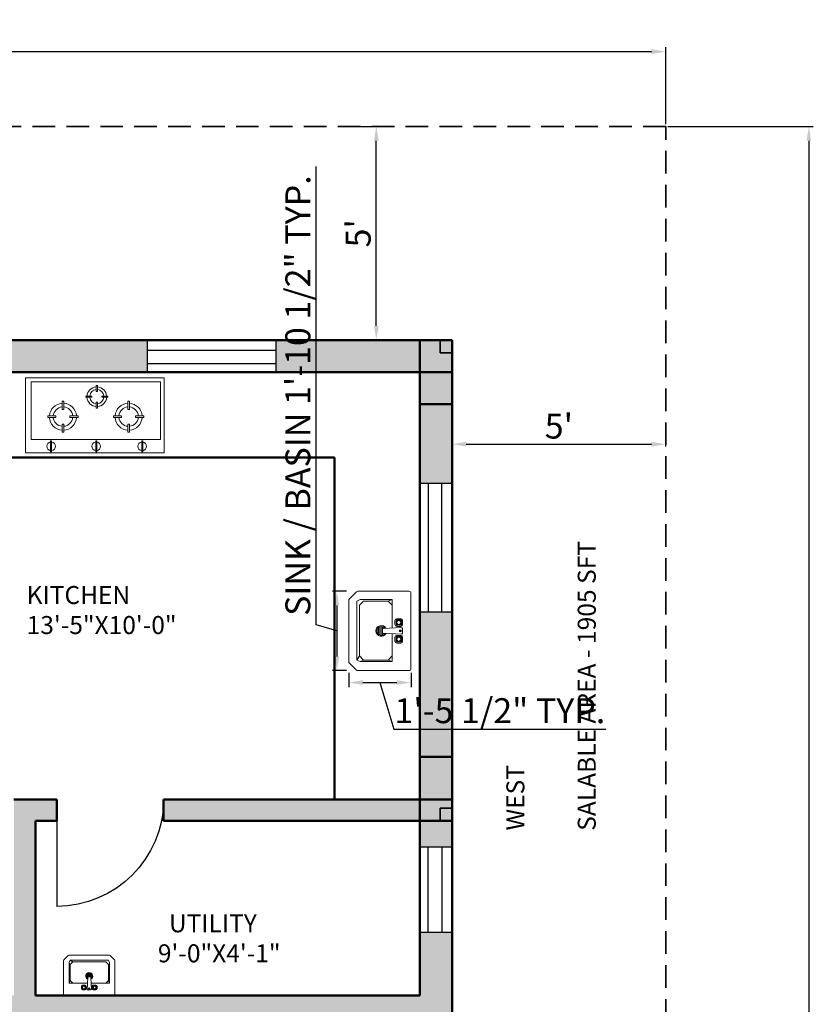
# Model space of a CAD drawing. Units: inches. Extents: x -7 to 1228, y -146 to 1091.
# Tile 88 of 88: x 1006 to 1228, y 814 to 1091. Entities that reach past the tile are written whole.
import ezdxf

# ---------------------------------------------------------------- set-up
doc = ezdxf.new("R2010")
doc.units = ezdxf.units.IN
doc.linetypes.add('DASHED2', pattern=[9.525, 6.35, -3.175])
for name, color, linetype, lineweight in [('A-ANNO-DIMS', 2, 'Continuous', 18), ('A-ANNO-TEXT', 7, 'Continuous', 18), ('A-AREA-IDEN', 7, 'Continuous', 18), ('A-COLS', 6, 'Continuous', 35), ('A-DOOR', 4, 'Continuous', 25), ('A-FURN', 8, 'Continuous', 18), ('A-GLAZ', 175, 'Continuous', 25), ('A-WALL', 7, 'Continuous', 50), ('A-WALL-PATT', 251, 'Continuous', 13), ('C-PROP', 1, 'DASHED2', 35)]:
    doc.layers.add(name, color=color, linetype=linetype, lineweight=lineweight)
doc.styles.get("Standard").update_dxf_attribs({"font": 'arial.ttf'})
doc.dimstyles.new('ISO-25', dxfattribs={"dimtxt": 7, "dimasz": 4, "dimexe": 1.25, "dimexo": 0.625, "dimtad": 1, "dimdec": 1, "dimlunit": 3, "dimtxsty": 'Standard', "dimcen": 2.5, "dimadec": 0, "dimazin": 0, "dimtfac": 1, "dimtdec": 1, "dimtmove": 1, "dimatfit": 3, "dimfxl": 1, "dimarcsym": 0})

# ---------------------------------------------------------------- blocks, each defined once
blk = doc.blocks.new('A$C72243D80')
at = {"ltscale": 1000}
for p, q in [((0, 0), (0, 384.2)), ((0, 384.2), (712, 384.2)), ((29.5, 68.9), (29.5, 363.2)), ((29.5, 363.2), (692.7, 363.2)), ((692.7, 363.2), (692.7, 68.9)), ((712, 384.2), (712, 0)), ((363.5, 314.5), (363.5, 345.1)), ((363.5, 345.1), (369.5, 345.1)), ((369.5, 314.5), (363.5, 314.5)), ((369.5, 345.1), (369.5, 314.5)), ((188.1, 264.2), (188.1, 222.1)), ((196.4, 264.2), (188.1, 264.2)), ((196.4, 222.1), (196.4, 264.2)), ((309.4, 291), (340, 291)), ((309.4, 285), (309.4, 291)), ((340, 285), (309.4, 285)), ((340, 291), (340, 285)), ((363.5, 260), (363.5, 229.4)), ((369.5, 260), (363.5, 260)), ((369.5, 229.4), (369.5, 260)), ((392.3, 291), (392.3, 285)), ((422.9, 291), (392.3, 291)), ((392.3, 285), (422.9, 285)), ((422.9, 285), (422.9, 291)), ((525.9, 222.1), (525.9, 264.2)), ((525.9, 264.2), (534.1, 264.2)), ((534.1, 264.2), (534.1, 222.1)), ((188.1, 222.1), (196.4, 222.1)), ((363.5, 229.4), (369.5, 229.4)), ((534.1, 222.1), (525.9, 222.1)), ((114.7, 189.8), (156.8, 189.8)), ((114.7, 181.6), (114.7, 189.8)), ((156.8, 181.6), (114.7, 181.6)), ((156.8, 189.8), (156.8, 181.6)), ((228.6, 189.8), (228.6, 181.6)), ((270.7, 189.8), (228.6, 189.8)), ((228.6, 181.6), (270.7, 181.6)), ((270.7, 181.6), (270.7, 189.8)), ((451.5, 189.8), (493.6, 189.8)), ((451.5, 181.6), (451.5, 189.8)), ((493.6, 181.6), (451.5, 181.6)), ((493.6, 189.8), (493.6, 181.6)), ((565.5, 189.8), (565.5, 181.6)), ((607.6, 189.8), (565.5, 189.8)), ((565.5, 181.6), (607.6, 181.6)), ((607.6, 181.6), (607.6, 189.8)), ((188.1, 147.2), (196.4, 147.2)), ((188.1, 105.1), (188.1, 147.2)), ((196.4, 105.1), (188.1, 105.1)), ((196.4, 147.2), (196.4, 105.1)), ((525.9, 147.2), (525.9, 105.1)), ((534.1, 147.2), (525.9, 147.2)), ((525.9, 105.1), (534.1, 105.1)), ((534.1, 105.1), (534.1, 147.2)), ((692.7, 68.9), (29.5, 68.9)), ((129.6, 61.1), (129.6, 5)), ((134.4, 61.1), (129.6, 61.1)), ((134.4, 5), (134.4, 61.1)), ((360.9, 5), (360.9, 61.1)), ((360.9, 61.1), (365.7, 61.1)), ((365.7, 61.1), (365.7, 5)), ((597, 5), (597, 61.1)), ((597, 61.1), (601.8, 61.1)), ((601.8, 61.1), (601.8, 5)), ((712, 0), (0, 0)), ((129.6, 5), (134.4, 5)), ((365.7, 5), (360.9, 5)), ((601.8, 5), (597, 5))]:
    blk.add_line(p, q, dxfattribs=at)
for centre, radius, start, end in [((366.2, 287.2), 50.3, 93.0344, 175.7271), ((366.1, 287.8), 36.3, 94.0374, 175.0142), ((366.2, 287.2), 50.3, 4.2729, 86.1838), ((366.1, 287.8), 36.3, 4.9858, 84.5356), ((192.7, 184.7), 69.2, 93.8162, 175.7271), ((192.7, 184.7), 69.2, 4.2729, 86.9656), ((366.2, 287.2), 50.3, 182.5783, 266.9656), ((366.1, 287.8), 36.3, 184.5153, 265.9626), ((366.1, 287.8), 36.3, 275.4644, 355.4847), ((366.2, 287.2), 50.3, 273.8162, 357.4217), ((529.5, 184.7), 69.2, 93.0344, 175.7271), ((529.5, 184.7), 69.2, 4.2729, 86.1838), ((192.9, 185.5), 49.9, 95.4644, 175.0142), ((192.9, 185.5), 49.9, 4.9858, 85.9626), ((529.4, 185.5), 49.9, 94.0374, 175.0142), ((529.4, 185.5), 49.9, 4.9858, 84.5356), ((192.7, 184.7), 69.2, 182.5783, 266.1838), ((192.9, 185.5), 49.9, 184.5153, 264.5356), ((192.9, 185.5), 49.9, 274.0374, 355.4847), ((192.7, 184.7), 69.2, 273.0344, 357.4217), ((529.5, 184.7), 69.2, 182.5783, 266.9656), ((529.4, 185.5), 49.9, 184.5153, 265.9626), ((529.5, 184.7), 69.2, 273.8162, 357.4217), ((529.4, 185.5), 49.9, 275.4644, 355.4847), ((132.3, 33.2), 22.5, 96.7453, 263.2547), ((132.3, 33.2), 22.5, 275.4789, 84.5211), ((363.1, 33.2), 22.5, 95.4789, 264.5211), ((363.1, 33.2), 22.5, 276.7453, 83.2547), ((599.2, 33.2), 22.5, 95.4789, 264.5211), ((599.2, 33.2), 22.5, 276.7453, 83.2547)]:
    blk.add_arc(centre, radius, start, end, dxfattribs=at)
blk = doc.blocks.new('A$C4CB854FF')
for p, q in [((0, 0.3675), (0, 0.0552)), ((0.4725, 0.38), (0.0125, 0.38)), ((0.485, 0.0552), (0.485, 0.3675)), ((0.1677, 0.2932), (0.1677, 0.318)), ((0.1745, 0.2919), (0.1745, 0.3194)), ((0.1773, 0.3221), (0.2048, 0.3221)), ((0.1787, 0.329), (0.2034, 0.329)), ((0.2075, 0.3194), (0.2075, 0.2919)), ((0.2144, 0.318), (0.2144, 0.2932)), ((0.2279, 0.2104), (0.2213, 0.3235)), ((0.2337, 0.329), (0.2502, 0.329)), ((0.2625, 0.3235), (0.256, 0.2104)), ((0.2694, 0.318), (0.2694, 0.2932)), ((0.2763, 0.3194), (0.2763, 0.2919)), ((0.3065, 0.3221), (0.279, 0.3221)), ((0.3052, 0.329), (0.2804, 0.329)), ((0.3093, 0.2919), (0.3093, 0.3194)), ((0.3162, 0.2932), (0.3162, 0.318)), ((0.05, 0.265), (0.2247, 0.265)), ((0.06, 0.24), (0.05, 0.265)), ((0.05, 0.07), (0.05, 0.265)), ((0.085, 0.265), (0.06, 0.24)), ((0.2048, 0.2891), (0.1773, 0.2891)), ((0.2034, 0.2822), (0.1787, 0.2822)), ((0.2591, 0.265), (0.43, 0.265)), ((0.279, 0.2891), (0.3065, 0.2891)), ((0.2804, 0.2822), (0.3052, 0.2822)), ((0.395, 0.265), (0.42, 0.24)), ((0.42, 0.24), (0.43, 0.265)), ((0.43, 0.07), (0.43, 0.265)), ((0.06, 0.24), (0.06, 0.09)), ((0.2152, 0.1984), (0.2694, 0.1984)), ((0.2297, 0.2066), (0.2165, 0.2066)), ((0.2681, 0.1901), (0.2165, 0.1901)), ((0.2272, 0.2149), (0.2208, 0.2149)), ((0.2638, 0.1819), (0.2208, 0.1819)), ((0.2505, 0.2052), (0.2334, 0.2052)), ((0.2681, 0.2066), (0.2541, 0.2066)), ((0.2638, 0.2149), (0.2566, 0.2149)), ((0.42, 0.24), (0.42, 0.09)), ((0.2533, 0.1736), (0.2313, 0.1736)), ((0.05, 0.07), (0.06, 0.05)), ((0.06, 0.09), (0.085, 0.065)), ((0.085, 0.065), (0.395, 0.065)), ((0.42, 0.09), (0.395, 0.065)), ((0.395, 0.065), (0.42, 0.05)), ((0.42, 0.09), (0.43, 0.07)), ((0.43, 0.07), (0.42, 0.05)), ((0.0037, 0.0463), (0.0463, 0.0037)), ((0.42, 0.05), (0.06, 0.05)), ((0.4387, 0.0037), (0.4813, 0.0463)), ((0.0552, 0), (0.4298, 0))]:
    blk.add_line(p, q)
for centre, radius in [((0.191, 0.3056), 0.0165), ((0.191, 0.3056), 0.0127), ((0.2419, 0.3152), 0.00688), ((0.2419, 0.3152), 0.00344), ((0.2928, 0.3056), 0.0165), ((0.2928, 0.3056), 0.0127)]:
    blk.add_circle(centre, radius)
for centre, radius, start, end in [((0.0125, 0.3675), 0.0125, 90, 180), ((0.4725, 0.3675), 0.0125, 0, 90), ((0.1787, 0.318), 0.011, 90, 180), ((0.1773, 0.3194), 0.00275, 90, 180), ((0.2034, 0.318), 0.011, 0, 90), ((0.2048, 0.3194), 0.00275, 360, 90), ((0.2329, 0.314), 0.015, 87.19754, 140.72744), ((0.2509, 0.314), 0.015, 39.27256, 92.80246), ((0.2804, 0.318), 0.011, 90, 180), ((0.279, 0.3194), 0.00275, 90, 180), ((0.3052, 0.318), 0.011, 0, 90), ((0.3065, 0.3194), 0.00275, 360, 90), ((0.1787, 0.2932), 0.011, 180, 270), ((0.1773, 0.2919), 0.00275, 180, 270), ((0.2034, 0.2932), 0.011, 270, 0), ((0.2048, 0.2919), 0.00275, 270, 0), ((0.2804, 0.2932), 0.011, 180, 270), ((0.279, 0.2919), 0.00275, 180, 270), ((0.3052, 0.2932), 0.011, 270, 360), ((0.3065, 0.2919), 0.00275, 270, 0), ((0.2423, 0.1984), 0.033, 118.68833, 62.86857), ((0.2423, 0.1984), 0.0271, 124.77581, 57.22467), ((0.2334, 0.2107), 0.0055, 183.3274, 270), ((0.2505, 0.2107), 0.0055, 270, 356.6726), ((0.0125, 0.0552), 0.0125, 180, 225), ((0.0552, 0.0125), 0.0125, 225, 270), ((0.4298, 0.0125), 0.0125, 270, 315), ((0.4725, 0.0552), 0.0125, 315, 0)]:
    blk.add_arc(centre, radius, start, end)
blk = doc.blocks.new('*D7')
at = {"layer": 'A-ANNO-DIMS', "color": 0, "lineweight": -2, "transparency": 16777216}
for p, q in [((1099.01, 1061), (1106.99, 1061)), ((1105.74, 1005), (1105.74, 1057)), ((1099.01, 1001), (1106.99, 1001))]:
    blk.add_line(p, q, dxfattribs=at)
at = {"layer": 'A-ANNO-DIMS', "color": 0, "transparency": 16777216}
for points in [[(1105.08, 1057), (1106.41, 1057), (1105.74, 1061)], [(1105.08, 1005), (1106.41, 1005), (1105.74, 1001)]]:
    blk.add_solid(points, dxfattribs=at)
at = {"layer": 'Defpoints', "color": 0, "transparency": 16777216}
for p in [(1098.39, 1061), (1105.74, 1061), (1098.39, 1001)]:
    blk.add_point(p, dxfattribs=at)
at = {"layer": 'A-ANNO-DIMS', "color": 0, "transparency": 16777216, "insert": (1101.56, 1031), "char_height": 7, "attachment_point": 5, "rotation": 90}
blk.add_mtext("5'", dxfattribs=at)
blk = doc.blocks.new('*D8')
at = {"layer": 'A-ANNO-DIMS', "color": 0, "lineweight": -2, "transparency": 16777216}
for p, q in [((1127, 971.1), (1127, 973.02)), ((1131, 971.77), (1183, 971.77)), ((1187, 971.1), (1187, 973.02))]:
    blk.add_line(p, q, dxfattribs=at)
at = {"layer": 'A-ANNO-DIMS', "color": 0, "transparency": 16777216}
for points in [[(1131, 972.44), (1131, 971.1), (1127, 971.77)], [(1183, 972.44), (1183, 971.1), (1187, 971.77)]]:
    blk.add_solid(points, dxfattribs=at)
at = {"layer": 'Defpoints', "color": 0, "transparency": 16777216}
for p in [(1127, 970.48), (1187, 971.77), (1187, 970.48)]:
    blk.add_point(p, dxfattribs=at)
at = {"layer": 'A-ANNO-DIMS', "color": 0, "transparency": 16777216, "insert": (1157, 975.95), "char_height": 7, "attachment_point": 5}
blk.add_mtext("5'", dxfattribs=at)
blk = doc.blocks.new('*D11')
at = {"layer": 'A-ANNO-DIMS', "color": 0, "lineweight": -2, "transparency": 16777216}
for p, q in [((0, 1061.62), (0, 1083.25)), ((4, 1082), (1183, 1082)), ((1187, 1061.62), (1187, 1083.25))]:
    blk.add_line(p, q, dxfattribs=at)
at = {"layer": 'A-ANNO-DIMS', "color": 0, "transparency": 16777216}
for points in [[(4, 1082.67), (4, 1081.33), (0, 1082)], [(1183, 1082.67), (1183, 1081.33), (1187, 1082)]]:
    blk.add_solid(points, dxfattribs=at)
at = {"layer": 'Defpoints', "color": 0, "transparency": 16777216}
for p in [(1187, 1082), (0, 1061), (1187, 1061)]:
    blk.add_point(p, dxfattribs=at)
at = {"layer": 'A-ANNO-DIMS', "color": 0, "transparency": 16777216, "insert": (593.5, 1086.2), "char_height": 7, "attachment_point": 5}
blk.add_mtext('98\'-11"', dxfattribs=at)
blk = doc.blocks.new('*D12')
at = {"layer": 'A-ANNO-DIMS', "color": 0, "lineweight": -2, "transparency": 16777216}
for p, q in [((1187.62, 1061), (1228.45, 1061)), ((1227.2, 1057), (1227.2, 4)), ((1187.62, 0), (1228.45, 0))]:
    blk.add_line(p, q, dxfattribs=at)
at = {"layer": 'A-ANNO-DIMS', "color": 0, "transparency": 16777216}
for points in [[(1226.53, 1057), (1227.86, 1057), (1227.2, 1061)], [(1226.53, 4), (1227.86, 4), (1227.2, 0)]]:
    blk.add_solid(points, dxfattribs=at)
at = {"layer": 'Defpoints', "color": 0, "transparency": 16777216}
for p in [(1187, 1061), (1187, 0), (1227.2, 0)]:
    blk.add_point(p, dxfattribs=at)
at = {"layer": 'A-ANNO-DIMS', "color": 0, "transparency": 16777216, "insert": (1223, 530.5), "char_height": 7, "attachment_point": 5, "rotation": 90}
blk.add_mtext('88\'-5"', dxfattribs=at)
blk = doc.blocks.new('WIN-36')
for p, q in [((0, 36), (0, 0)), ((9, 36), (0, 36)), ((2.34, 36), (2.34, 0)), ((6.14, 0), (6.14, 36)), ((9, 0), (9, 36)), ((0, 0), (9, 0)), ((2.34, 0), (6.14, 0))]:
    blk.add_line(p, q)
blk = doc.blocks.new('WIN-24')
for p, q in [((0, 0), (0, 24)), ((0, 24), (9, 24)), ((2.34, 0), (2.34, 24)), ((2.34, 24), (6.14, 24)), ((6.14, 24), (6.14, 0)), ((9, 24), (9, 0)), ((9, 0), (0, 0))]:
    blk.add_line(p, q)
blk = doc.blocks.new('DOOR-750')
blk.add_line((30, 30), (30, 0))
blk.add_arc((30, 30), 30, 180, 270)
blk = doc.blocks.new('*D30')
at = {"layer": 'A-ANNO-DIMS', "color": 0, "lineweight": -2, "transparency": 16777216}
for p, q in [((1088.85, 921.08), (1088.85, 1049.76)), ((1097.38, 930.49), (1093.41, 930.49)), ((1094.66, 926.49), (1094.66, 912.19)), ((1094.66, 919.34), (1088.85, 921.08)), ((1097.38, 908.19), (1093.41, 908.19))]:
    blk.add_line(p, q, dxfattribs=at)
at = {"layer": 'A-ANNO-DIMS', "color": 0, "transparency": 16777216}
for points in [[(1093.99, 926.49), (1095.32, 926.49), (1094.66, 930.49)], [(1093.99, 912.19), (1095.32, 912.19), (1094.66, 908.19)]]:
    blk.add_solid(points, dxfattribs=at)
at = {"layer": 'Defpoints', "color": 0, "transparency": 16777216}
for p in [(1098, 930.49), (1094.66, 908.19), (1098, 908.19)]:
    blk.add_point(p, dxfattribs=at)
at = {"layer": 'A-ANNO-DIMS', "color": 0, "transparency": 16777216, "insert": (1084.61, 985.42), "char_height": 7, "attachment_point": 5, "rotation": 90}
blk.add_mtext('SINK / BASIN 1\'-10 1/2" TYP.', dxfattribs=at)
blk = doc.blocks.new('*D31')
at = {"layer": 'A-ANNO-DIMS', "color": 0, "lineweight": -2, "transparency": 16777216}
for p, q in [((1098, 907.56), (1098, 903.59)), ((1115.48, 907.56), (1115.48, 903.59)), ((1102, 904.84), (1111.48, 904.84)), ((1106.74, 904.84), (1110.66, 891.8)), ((1110.66, 891.8), (1170.23, 891.8))]:
    blk.add_line(p, q, dxfattribs=at)
at = {"layer": 'A-ANNO-DIMS', "color": 0, "transparency": 16777216}
for points in [[(1102, 905.51), (1102, 904.18), (1098, 904.84)], [(1111.48, 905.51), (1111.48, 904.18), (1115.48, 904.84)]]:
    blk.add_solid(points, dxfattribs=at)
at = {"layer": 'Defpoints', "color": 0, "transparency": 16777216}
for p in [(1098, 908.19), (1115.48, 908.19), (1115.48, 904.84)]:
    blk.add_point(p, dxfattribs=at)
at = {"layer": 'A-ANNO-DIMS', "color": 0, "transparency": 16777216, "insert": (1140.44, 896.04), "char_height": 7, "attachment_point": 5}
blk.add_mtext('1\'-5 1/2" TYP.', dxfattribs=at)

msp = doc.modelspace()

# ---------------------------------------------------------------- hatches: boundary and pattern name
at = {"layer": 'A-COLS'}
h = msp.add_hatch(color=256, dxfattribs=at)
h.dxf.hatch_style = 1
h.paths.add_polyline_path([(1127, 997.45), (1123.71, 997.45), (1123.71, 1001), (1118, 1001), (1118, 983), (1127, 983)])
h = msp.add_hatch(color=256, dxfattribs=at)
h.dxf.hatch_style = 1
h.paths.add_polyline_path([(1127, 997.45), (1127, 1001), (1123.71, 1001), (1123.71, 997.45)])
h = msp.add_hatch(color=256, dxfattribs=at)
h.dxf.hatch_style = 1
h.paths.add_polyline_path([(1127, 884), (1118, 884), (1118, 866), (1123.71, 866), (1123.71, 869.55), (1127, 869.55)])
h = msp.add_hatch(color=256, dxfattribs=at)
h.dxf.hatch_style = 1
h.paths.add_polyline_path([(1123.71, 869.55), (1123.71, 866), (1127, 866), (1127, 869.55)])
at = {"layer": 'A-WALL-PATT'}
h = msp.add_hatch(color=256, dxfattribs=at)
h.dxf.hatch_style = 1
h.paths.add_polyline_path([(69, 568), (60, 568), (60, 493), (63.29, 493), (69, 493)])
h.paths.add_polyline_path([(69, 662.41), (60, 662.41), (60, 586), (69, 586)], flags=17)
h.paths.add_polyline_path([(69, 723), (184, 723), (184, 734), (179, 734), (179, 728), (69, 728), (69, 741.62), (60, 741.62), (60, 698.41), (69, 698.41)], flags=17)
h.paths.add_polyline_path([(69, 782), (231, 782), (231, 728), (231, 723), (231, 586), (236, 586), (236, 787), (69, 787), (69, 800.13), (60, 800.13), (60, 765.62), (69, 765.62)])
h.paths.add_polyline_path([(184, 842), (189, 842), (189, 848), (173, 848), (173, 842), (179, 842), (179, 787), (184, 787)])
h.paths.add_polyline_path([(118.22, 69), (69, 69), (69, 60), (118.22, 60)])
h.paths.add_polyline_path([(227, 69), (154.22, 69), (154.22, 60), (227, 60)])
h.paths.add_polyline_path([(236, 60), (232.71, 60), (227, 60), (227, 36), (236, 36)])
h.paths.add_polyline_path([(389, 60), (380, 60), (380, 36), (389, 36)])
h.paths.add_polyline_path([(384, 181), (380, 181), (380, 115), (380, 78), (384, 78)])
h.paths.add_polyline_path([(380, 115), (334.55, 115), (334.55, 109), (380, 109)])
h.paths.add_polyline_path([(274.55, 115), (236, 115), (236, 201), (232.71, 201), (231, 201), (231, 78), (236, 78), (236, 109), (274.55, 109)])
h.paths.add_polyline_path([(69, 123), (60, 123), (60, 78), (69, 78)])
h.paths.add_polyline_path([(69, 201), (60, 201), (60, 159), (69, 159)])
h.paths.add_polyline_path([(143, 219), (69, 219), (69, 213), (143, 213)], flags=17)
h.paths.add_polyline_path([(189, 219), (184, 219), (184, 274), (231, 274), (231, 219), (236, 219), (236, 279), (184, 279), (184, 297), (179, 297), (179, 279), (69, 279), (69, 290.91), (60, 290.91), (60, 262.18), (69, 262.18), (69, 274), (179, 274), (179, 219), (173, 219), (173, 213), (189, 213)])
h.paths.add_polyline_path([(69, 238.18), (60, 238.18), (60, 219), (69, 219)], flags=17)
h.paths.add_polyline_path([(69, 333), (60, 333), (60, 314.91), (69, 314.91), (69, 316.96)])
h.paths.add_polyline_path([(190, 338), (184, 338), (69, 338), (69, 333), (179, 333), (179, 327), (184, 327), (184, 333.02), (190, 333.05)])
h.paths.add_polyline_path([(69, 386.81), (60, 386.81), (60, 351), (69, 351)])
h.paths.add_polyline_path([(69, 475), (60, 475), (60, 422.81), (69, 422.81)])
h.paths.add_polyline_path([(236, 475), (231, 475), (231, 351.24), (236, 351.24)])
h.paths.add_polyline_path([(384, 475), (380, 475), (380, 362), (384, 362)])
h.paths.add_polyline_path([(547, 307), (439, 307), (439, 356), (445, 356), (445, 362), (433, 362), (433, 307), (380, 307), (380, 244), (380, 241), (384, 241), (384, 301), (433, 301), (433, 277), (439, 277), (439, 301), (547, 301)])
h.paths.add_polyline_path([(547, 241), (439, 241), (439, 247), (433, 247), (433, 235), (547, 235)])
h.paths.add_polyline_path([(450, 69), (440.29, 69), (424.89, 69), (389, 69), (389, 60), (450, 60)])
h.paths.add_polyline_path([(547, 69), (486, 69), (486, 60), (547, 60)])
h.paths.add_polyline_path([(556, 148.27), (547, 148.27), (547, 78), (556, 78)])
h.paths.add_polyline_path([(556, 223), (547, 223), (547, 195), (547, 184.27), (556, 184.27)])
h.paths.add_polyline_path([(556, 311.19), (547, 311.19), (547, 273.08), (556, 273.08)])
h.paths.add_polyline_path([(556, 344), (552.71, 344), (547, 344), (547, 335.19), (556, 335.19)])
h.paths.add_polyline_path([(556, 249.08), (547, 249.08), (547, 241), (556, 241)])
h.paths.add_polyline_path([(547, 362), (475, 362), (475, 356), (547, 356)], flags=0)
h.paths.add_polyline_path([(556, 399.62), (547, 399.62), (547, 362), (556, 362)])
h.paths.add_polyline_path([(556, 475), (547, 475), (547, 435.62), (556, 435.62)])
h.paths.add_polyline_path([(547, 493), (389, 493), (389, 487), (547, 487)])
h.paths.add_polyline_path([(380, 493), (278, 493), (278, 487), (380, 487)])
h.paths.add_polyline_path([(227, 493), (69, 493), (69, 487), (227, 487)])
h.paths.add_polyline_path([(643, 122.44), (634, 122.44), (634, 78), (643, 78)])
h.paths.add_polyline_path([(702.5, 69), (692.79, 69), (677.39, 69), (643, 69), (643, 60), (702.5, 60)])
h.paths.add_polyline_path([(798, 69), (738.5, 69), (738.5, 60), (798, 60)])
h.paths.add_polyline_path([(807, 60), (803.71, 60), (798, 60), (798, 36), (807, 36)])
h.paths.add_polyline_path([(807, 109), (846.75, 109), (846.75, 115), (807, 115), (807, 159), (802, 159), (802, 78), (807, 78)])
h.paths.add_polyline_path([(807, 201), (802, 201), (802, 195), (807, 195)])
h.paths.add_polyline_path([(643, 201), (634, 201), (634, 158.44), (643, 158.44)])
h.paths.add_polyline_path([(756, 225), (751, 225), (751, 219), (643, 219), (643, 213), (756, 213)])
h.paths.add_polyline_path([(643, 240.85), (634, 240.85), (634, 219), (643, 219)])
h.paths.add_polyline_path([(643, 274), (643, 288.63), (634, 288.63), (634, 264.85), (643, 264.85)])
h.paths.add_polyline_path([(802, 279), (756, 279), (756, 297), (751, 297), (751, 279), (643, 279), (643, 274), (751, 274), (751, 255), (756, 255), (756, 274), (802, 274)])
h.paths.add_polyline_path([(807, 333), (803.71, 333), (802, 333), (802, 279), (802, 274), (802, 219), (807, 219)])
h.paths.add_polyline_path([(956, 182), (951, 182), (951, 115), (906.75, 115), (906.75, 109), (951, 109), (951, 78), (956, 78)])
h.paths.add_polyline_path([(960, 60), (951, 60), (951, 36), (960, 36)])
h.paths.add_polyline_path([(1021, 69), (1005.78, 69), (960, 69), (960, 60), (1021, 60)])
h.paths.add_polyline_path([(956, 224), (951, 224), (951, 218), (956, 218)])
h.paths.add_polyline_path([(956, 302), (1004, 302), (1004, 278), (1010, 278), (1010, 302), (1118, 302), (1118, 290.81), (1127, 290.81), (1127, 326.97), (1118, 326.97), (1118, 320.97), (1118, 307), (1010, 307), (1010, 356), (1016, 356), (1016, 362), (1004, 362), (1004, 307), (951, 307), (951, 244), (951, 242), (954.29, 242), (956, 242)])
h.paths.add_polyline_path([(643, 333), (634, 333), (634, 312.63), (643, 312.63), (643, 316.96)])
h.paths.add_polyline_path([(756, 338), (643, 338), (643, 333), (751, 333), (751, 327), (756, 327)])
h.paths.add_polyline_path([(643, 388), (634, 388), (634, 351), (643, 351)])
h.paths.add_polyline_path([(807, 357), (802, 357), (802, 351), (807, 351)])
h.paths.add_polyline_path([(807, 475), (802, 475), (802, 393), (807, 393)])
h.paths.add_polyline_path([(643, 475), (634, 475), (634, 424), (643, 424)])
h.paths.add_polyline_path([(798, 493), (643, 493), (643, 487), (798, 487)])
h.paths.add_polyline_path([(634, 493), (556, 493), (556, 487), (634, 487)])
h.paths.add_polyline_path([(813, 493), (807, 493), (807, 487), (813, 487)])
h.paths.add_polyline_path([(951, 493), (849, 493), (849, 487), (951, 487)])
h.paths.add_polyline_path([(956, 484), (951, 484), (951, 374), (956, 374)])
h.paths.add_polyline_path([(1109, 493), (969, 493), (969, 487), (1109, 487)])
h.paths.add_polyline_path([(1127, 484), (1118, 484), (1118, 450.64), (1127, 450.64)])
h.paths.add_polyline_path([(1127, 414.64), (1118, 414.64), (1118, 365), (1127, 365)])
h.paths.add_polyline_path([(1109, 362), (1046, 362), (1046, 356), (1109, 356)], flags=17)
h.paths.add_polyline_path([(1127, 356), (1123.45, 356), (1118, 356), (1118, 350.97), (1127, 350.97)], flags=0)
h.paths.add_polyline_path([(1127, 266.81), (1118, 266.81), (1118, 262.36), (1118, 242), (1127, 242)], flags=17)
h.paths.add_polyline_path([(1118, 242), (1010, 242), (1010, 248), (1004, 248), (1004, 237), (1118, 237)])
h.paths.add_polyline_path([(1127, 224), (1118, 224), (1118, 170), (1127, 170)])
h.paths.add_polyline_path([(1127, 134), (1118, 134), (1118, 78), (1127, 78)])
h.paths.add_polyline_path([(1118, 69), (1057, 69), (1057, 60), (1118, 60)])
h.paths.add_polyline_path([(227, 571.55), (227, 574), (69, 574), (69, 568), (227, 568)])
h.paths.add_polyline_path([(380, 571.55), (380, 574), (278, 574), (278, 568), (380, 568)])
h.paths.add_polyline_path([(242, 574), (236, 574), (236, 568), (242, 568)])
h.paths.add_polyline_path([(547, 571.55), (547, 574), (389, 574), (389, 568), (547, 568)])
h.paths.add_polyline_path([(384, 733), (380, 733), (380, 586), (384, 586)])
h.paths.add_polyline_path([(556, 646), (634, 646), (634, 655), (547, 655), (547, 586), (556, 586)])
h.paths.add_polyline_path([(634, 574), (556, 574), (556, 568), (634, 568)])
h.paths.add_polyline_path([(643, 655), (634, 655), (634, 586), (643, 586)])
h.paths.add_polyline_path([(798, 574), (643, 574), (643, 568), (798, 568)])
h.paths.add_polyline_path([(643, 663.85), (634, 663.85), (634, 655), (643, 655)])
h.paths.add_polyline_path([(556, 676.97), (547, 676.97), (547, 655), (556, 655)])
h.paths.add_polyline_path([(556, 733), (547, 733), (547, 712.97), (556, 712.97)])
h.paths.add_polyline_path([(643, 710), (634, 710), (634, 699.85), (643, 699.85)])
h.paths.add_polyline_path([(807, 668), (802, 668), (802, 586), (807, 586)])
h.paths.add_polyline_path([(951, 574), (849, 574), (849, 568), (951, 568)])
h.paths.add_polyline_path([(956, 691), (951, 691), (951, 577), (956, 577)])
h.paths.add_polyline_path([(1109, 574), (969, 574), (969, 568), (1109, 568)])
h.paths.add_polyline_path([(1127, 643.4), (1118, 643.4), (1118, 577), (1127, 577)])
h.paths.add_polyline_path([(1127, 568), (1123.45, 568), (1118, 568), (1118, 493), (1127, 493)])
h.paths.add_polyline_path([(1127, 733), (1118, 733), (1118, 679.4), (1127, 679.4)])
h.paths.add_polyline_path([(1127, 777.35), (1118, 777.35), (1118, 770.04), (1118, 751), (1127, 751)], flags=17)
h.paths.add_polyline_path([(1118, 751), (1010, 751), (1010, 757), (1004, 757), (1004, 745), (1118, 745)])
h.paths.add_polyline_path([(956, 811), (1004, 811), (1004, 787), (1010, 787), (1010, 811), (1017.87, 811), (1017.87, 811.63, -0.414214), (1018.25, 812), (1031.98, 812, -0.414214), (1032.35, 811.63), (1032.35, 811), (1118, 811), (1118, 801.35), (1127, 801.35), (1127, 834.69), (1118, 834.69), (1118, 830.24), (1118, 817), (1010, 817), (1010, 866), (1016, 866), (1016, 872), (1004, 872), (1004, 817), (956, 817), (956, 866), (951, 866), (951, 751), (954.29, 751), (956, 751)])
h.paths.add_polyline_path([(1118, 872), (1046, 872), (1046, 866), (1118, 866)], flags=17)
h.paths.add_polyline_path([(1127, 924.71), (1118, 924.71), (1118, 884), (1127, 884)])
h.paths.add_polyline_path([(1127, 866), (1123.71, 866), (1118, 866), (1118, 858.69), (1127, 858.69)], flags=17)
h.paths.add_polyline_path([(956, 983), (951, 983), (951, 952), (807, 952), (807, 983), (802, 983), (802, 902), (807, 902), (807, 946), (951, 946), (951, 884), (956, 884)])
h.paths.add_polyline_path([(807, 842), (802, 842), (802, 787), (756, 787), (756, 806), (751, 806), (751, 787), (643, 787), (643, 782), (751, 782), (751, 764), (756, 764), (756, 782), (802, 782), (802, 728), (807, 728)])
h.paths.add_polyline_path([(756, 848), (643, 848), (643, 842), (751, 842), (751, 836), (756, 836)])
h.paths.add_polyline_path([(756, 734), (751, 734), (751, 728), (643, 728), (643, 723), (756, 723)])
h.paths.add_polyline_path([(643, 749.79), (634, 749.79), (634, 728), (637.29, 728), (643, 728)])
h.paths.add_polyline_path([(643, 805.41), (634, 805.41), (634, 773.79), (643, 773.79)])
h.paths.add_polyline_path([(643, 896.66), (634, 896.66), (634, 860), (637.29, 860), (643, 860)])
h.paths.add_polyline_path([(643, 842), (634, 842), (634, 829.41), (643, 829.41)])
h.paths.add_polyline_path([(643, 983), (634, 983), (634, 932.66), (643, 932.66)])
h.paths.add_polyline_path([(1127, 983), (1118, 983), (1118, 960.71), (1127, 960.71)])
h.paths.add_polyline_path([(1118, 1001), (1077.53, 1001), (1077.53, 992), (1118, 992)])
h.paths.add_polyline_path([(1041.53, 1001), (960, 1001), (960, 992), (1041.53, 992)])
h.paths.add_polyline_path([(960, 1025), (951, 1025), (951, 1001), (954.29, 1001), (960, 1001)])
h.paths.add_polyline_path([(807, 1025), (798, 1025), (798, 1001), (807, 1001)])
h.paths.add_polyline_path([(798, 1001), (738.5, 1001), (738.5, 992), (798, 992)])
h.paths.add_polyline_path([(702.5, 1001), (643, 1001), (643, 992), (702.5, 992)])
h.paths.add_polyline_path([(547, 1001), (499.11, 1001), (499.11, 992), (547, 992)])
h.paths.add_polyline_path([(463.11, 1001), (389, 1001), (389, 992), (463.11, 992)])
h.paths.add_polyline_path([(389, 1025), (380, 1025), (380, 1022), (380, 1001), (383.29, 1001), (389, 1001)])
h.paths.add_polyline_path([(236, 1025), (227, 1025), (227, 1001), (236, 1001)])
h.paths.add_polyline_path([(236, 983), (231, 983), (231, 860), (236, 860)])
h.paths.add_polyline_path([(274.55, 952), (236, 952), (236, 946), (274.55, 946)])
h.paths.add_polyline_path([(380, 952), (334.55, 952), (334.55, 946), (380, 946)])
h.paths.add_polyline_path([(384, 983), (380, 983), (380, 884), (383.29, 884), (384, 884)])
h.paths.add_polyline_path([(227, 1001), (155.01, 1001), (155.01, 992), (162.87, 992), (227, 992)])
h.paths.add_polyline_path([(119.01, 1001), (69, 1001), (69, 992), (119.01, 992)])
h.paths.add_polyline_path([(69, 983), (60, 983), (60, 922.99), (69, 922.99)])
h.paths.add_polyline_path([(69, 886.99), (60, 886.99), (60, 860), (63.29, 860), (69, 860)])
h.paths.add_polyline_path([(143, 848), (69, 848), (69, 842), (143, 842)])

# ---------------------------------------------------------------- linework, layer by layer
at = {"layer": 'A-COLS'}
for points in [[(1127, 1001), (1123.71, 1001), (1123.71, 997.45), (1127, 997.45)], [(1127, 866), (1123.71, 866), (1123.71, 869.55), (1127, 869.55)]]:
    msp.add_lwpolyline(points, close=True, dxfattribs=at)
at = {"layer": 'A-WALL'}
for p, q in [((1127, 1001), (951, 1001)), ((1127, 1001), (1118, 1001)), ((1118, 1001), (1118, 983)), ((1118, 817), (1118, 1001)), ((1127, 60), (1127, 1001)), ((1127, 983), (1127, 1001)), ((1127, 992), (951, 992)), ((1118, 983), (1127, 983)), ((1094, 968), (956, 968)), ((1094, 872), (1094, 968)), ((1118, 866), (1118, 884)), ((1118, 884), (1127, 884)), ((1127, 884), (1127, 866)), ((1016, 872), (1004, 872)), ((1016, 866), (1016, 872)), ((1127, 872), (1046, 872)), ((1046, 866), (1046, 872)), ((1010, 817), (1010, 866)), ((1016, 866), (1010, 866)), ((1127, 866), (1046, 866)), ((1127, 866), (1118, 866)), ((1118, 817), (1010, 817))]:
    msp.add_line(p, q, dxfattribs=at)
at = {"layer": 'C-PROP'}
for p, q in [((1187, 1061), (0, 1061)), ((1187, 0), (1187, 1061))]:
    msp.add_line(p, q, dxfattribs=at)

# ---------------------------------------------------------------- block references
at = {"layer": 'A-DOOR', "extrusion": (0, 0, -1), "zscale": -1}
msp.add_blockref('DOOR-750', (-1046, 842), dxfattribs=at)
at = {"layer": 'A-FURN', "xscale": 0.0547573419986423, "yscale": 0.0547573419986423, "zscale": 0.0547573419986423}
msp.add_blockref('A$C72243D80', (1007.2, 969.36), dxfattribs=at)
at = {"layer": 'A-FURN'}
for p, xscale, yscale, zscale, rotation in [((1098, 930.49), 45.99182974636398, 45.99182974636398, 45.99182974636398, 270), ((1032.35, 828.34), 29.84864686937646, 29.84864686937646, 29.84864686937646, 180)]:
    msp.add_blockref('A$C4CB854FF', p, dxfattribs=dict(at, xscale=xscale, yscale=yscale, zscale=zscale, rotation=rotation))
at = {"layer": 'A-GLAZ', "extrusion": (0, 0, -1), "zscale": -1, "rotation": 89.99999999999994}
msp.add_blockref('WIN-36', (-1041.53, 992), dxfattribs=at)
at = {"layer": 'A-GLAZ'}
for name, p in [('WIN-36', (1118, 924.71)), ('WIN-24', (1118, 834.68))]:
    msp.add_blockref(name, p, dxfattribs=at)

# ---------------------------------------------------------------- texts
at = {"layer": 'A-ANNO-TEXT', "attachment_point": 1, "rotation": 90}
for s, insert, char_height in [('{SALABLE AREA - 1905 SFT}', (1162.3, 863.22), 5.0568), ('WEST', (1142.26, 863.31), 5.057)]:
    msp.add_mtext_dynamic_manual_height_columns(s, width=137.2821, gutter_width=25.28, heights=[0], dxfattribs=dict(at, insert=insert, char_height=char_height))
at = {"layer": 'A-AREA-IDEN', "char_height": 5.0568, "attachment_point": 1}
for s, insert in [(' KITCHEN\\P 13\'-5"X10\'-0"', (1006.01, 931.95)), ('  UTILITY\\P9\'-0"X4\'-1"', (1044.41, 839.77))]:
    msp.add_mtext_dynamic_manual_height_columns(s, width=137.2821, gutter_width=25.28, heights=[0], dxfattribs=dict(at, insert=insert))

# ---------------------------------------------------------------- dimensions: what is measured, and where the dimension line sits
at = {"layer": 'A-ANNO-DIMS'}
for base, p1, p2, picture, middle in [((1187, 1082), (0, 1061), (1187, 1061), '*D11', (593.5, 1086.2)), ((1187, 971.77), (1127, 970.48), (1187, 970.48), '*D8', (1157, 975.95))]:
    dim = msp.add_linear_dim(base=base, p1=p1, p2=p2, dimstyle='ISO-25', override={"dimclrd": 0, "dimclre": 0, "dimclrt": 0}, dxfattribs=at)
    dim.commit()
    dim.dimension.update_dxf_attribs({"geometry": picture, "text_midpoint": middle})
for base, p1, p2, picture, middle in [((1105.74, 1061), (1098.39, 1001), (1098.39, 1061), '*D7', (1101.56, 1031)), ((1227.2, 0), (1187, 1061), (1187, 0), '*D12', (1223, 530.5))]:
    dim = msp.add_linear_dim(base=base, p1=p1, p2=p2, angle=90, dimstyle='ISO-25', override={"dimclrd": 0, "dimclre": 0, "dimclrt": 0}, dxfattribs=at)
    dim.commit()
    dim.dimension.update_dxf_attribs({"geometry": picture, "text_midpoint": middle})
dim = msp.add_linear_dim(base=(1094.66, 908.19), p1=(1098, 930.49), p2=(1098, 908.19), angle=270, text='SINK / BASIN <> TYP.', dimstyle='ISO-25', override={"dimdec": 1, "dimlfac": 1, "dimrnd": 0, "dimzin": 1, "dimdsep": 46, "dimlunit": 4, "dimfrac": 2}, dxfattribs=at)
dim.commit()
dim.dimension.update_dxf_attribs({"geometry": '*D30', "text_midpoint": (1084.61, 921.71)})
dim = msp.add_linear_dim(base=(1115.48, 904.84), p1=(1098, 908.19), p2=(1115.48, 908.19), text='<> TYP.', dimstyle='ISO-25', override={"dimdec": 1, "dimlfac": 1, "dimrnd": 0, "dimzin": 1, "dimdsep": 46, "dimlunit": 4, "dimfrac": 2}, dxfattribs=at)
dim.commit()
dim.dimension.update_dxf_attribs({"geometry": '*D31', "text_midpoint": (1111.28, 896.04)})

doc.saveas('drawing.dxf')
